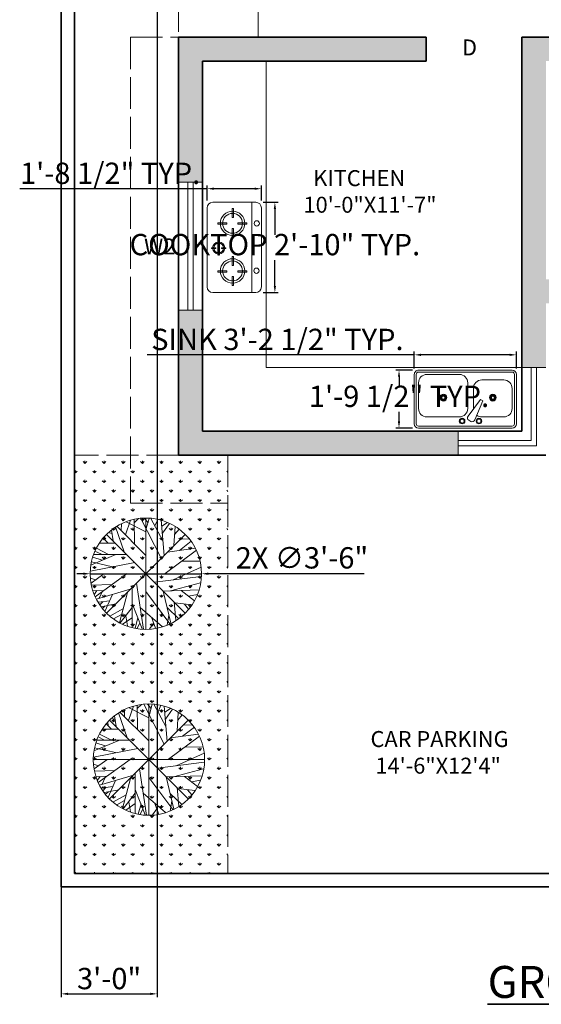
# Model space of a CAD drawing. Units: inches. Extents: x 1070 to 2371, y 645 to 1546.
# Tile 1 of 10: x 1147 to 1342, y 645 to 1014. Entities that reach past the tile are written whole.
import ezdxf

# ---------------------------------------------------------------- set-up
doc = ezdxf.new("R2010")
doc.units = ezdxf.units.IN
doc.linetypes.add('ACAD_ISO02W100', pattern=[15, 12, -3])
for name, color, linetype, lineweight in [('A-ANNO-DIMS', 2, 'Continuous', 18), ('A-ANNO-TEXT', 7, 'Continuous', 18), ('A-ANNO-TITL', 7, 'Continuous', 35), ('A-AREA-IDEN', 7, 'Continuous', 18), ('A-DOOR', 4, 'Continuous', 18), ('A-EQPM', 9, 'Continuous', 18), ('A-FLOR-CASE', 9, 'Continuous', 18), ('A-FLOR-FIXT', 9, 'Continuous', 18), ('A-GLAZ', 4, 'Continuous', 18), ('A-ROOF-OVHD', 8, 'ACAD_ISO02W100', 13), ('A-WALL', 7, 'Continuous', 35), ('C-PROP', 7, 'Continuous', 35), ('L-PLNT-BEDS-HIDN', 3, 'ACAD_ISO02W100', 13), ('L-PLNT-TREE', 94, 'Continuous', 13)]:
    doc.layers.add(name, color=color, linetype=linetype, lineweight=lineweight)
doc.layers.add('A-WALL-PATT', color=162, linetype='Continuous', lineweight=13, true_color=0x044ac3)
doc.layers.add('L-PLNT-PATT', color=85, linetype='Continuous', lineweight=13, true_color=0x58ba48)
doc.styles.get("Standard").update_dxf_attribs({"font": 'arial.ttf'})
doc.dimstyles.new('ISO-25', dxfattribs={"dimtxt": 8, "dimasz": 2.5, "dimexe": 1.25, "dimexo": 0.625, "dimtad": 1, "dimtih": 1, "dimtoh": 1, "dimdec": 1, "dimlunit": 3, "dimtxsty": 'Standard', "dimcen": 2.5, "dimadec": 0, "dimazin": 0, "dimtfac": 1, "dimtdec": 1, "dimtmove": 0, "dimatfit": 3, "dimfxl": 1, "dimarcsym": 0})

# ---------------------------------------------------------------- blocks, each defined once
blk = doc.blocks.new('A$C51B36FC3')
at = {"linetype": 'ByBlock'}
for p, q in [((0, 421.4), (0, 33)), ((15, 421.4), (15, 33)), ((767.9, 454.4), (33, 454.4)), ((767.9, 439.4), (33, 439.4)), ((325.7, 391), (261.9, 241.3)), ((357.3, 402.3), (372.7, 393.4)), ((785.9, 33), (785.9, 421.4)), ((800.9, 33), (800.9, 421.4)), ((99.1, 366.3), (271.4, 366.3)), ((281, 230.3), (378.7, 360.4)), ((447.6, 366.3), (701.8, 366.3)), ((33, 143.2), (33, 300.3)), ((171.7, 226.6), (164.2, 233.2)), ((174.6, 229.3), (168.8, 237.4)), ((178.2, 231.2), (174.5, 240.5)), ((181.4, 232.2), (179.7, 242)), ((185.3, 232.4), (185.8, 242.4)), ((189.3, 231.7), (192.3, 241.3)), ((193.1, 230.1), (198.2, 238.7)), ((196, 227.8), (203, 235)), ((261.9, 241.3), (281, 230.3)), ((337.5, 299.4), (337.5, 143.2)), ((381.5, 99.1), (381.5, 300.3)), ((560, 226.6), (552.4, 233.2)), ((562.9, 229.3), (557.1, 237.4)), ((566.5, 231.2), (562.8, 240.5)), ((569.7, 232.2), (567.9, 242)), ((573.5, 232.4), (574, 242.4)), ((577.6, 231.7), (580.5, 241.3)), ((581.3, 230.1), (586.4, 238.7)), ((584.3, 227.8), (591.2, 235)), ((767.9, 300.3), (767.9, 99.1)), ((167.7, 217.2), (157.7, 218.2)), ((167.7, 213.8), (157.8, 212.7)), ((168.5, 220.9), (159, 224.1)), ((168.6, 210), (159.2, 206.6)), ((169.7, 223.8), (161, 228.6)), ((170.1, 206.9), (161.5, 201.7)), ((172.4, 203.8), (165.3, 196.8)), ((175, 201.7), (169.3, 193.4)), ((179.3, 199.6), (176.3, 190.1)), ((184.7, 198.8), (184.8, 188.8)), ((188.6, 199.3), (191.1, 189.6)), ((192, 200.6), (196.5, 191.7)), ((195.5, 202.9), (202.1, 195.4)), ((198.3, 206.1), (206.6, 200.5)), ((199, 224.1), (207.6, 229.1)), ((200.1, 209.6), (209.5, 206)), ((200.4, 221), (209.9, 224.1)), ((201, 212.9), (210.9, 211.3)), ((201.2, 216.9), (211.2, 217.6)), ((555.9, 217.2), (546, 218.2)), ((556, 213.8), (546, 212.7)), ((556.7, 220.9), (547.2, 224.1)), ((556.8, 210), (547.4, 206.6)), ((558, 223.8), (549.2, 228.6)), ((558.3, 206.9), (549.8, 201.7)), ((560.7, 203.8), (553.6, 196.8)), ((563.2, 201.7), (557.6, 193.4)), ((567.6, 199.6), (564.5, 190.1)), ((572.9, 198.8), (573.1, 188.8)), ((576.9, 199.3), (579.4, 189.6)), ((580.3, 200.6), (584.8, 191.7)), ((583.7, 202.9), (590.3, 195.4)), ((586.6, 206.1), (594.8, 200.5)), ((587.2, 224.1), (595.9, 229.1)), ((588.4, 209.6), (597.7, 206)), ((588.6, 221), (598.1, 224.1)), ((589.3, 212.9), (599.2, 211.3)), ((589.5, 216.9), (599.4, 217.6)), ((33, 15), (767.9, 15)), ((33, 0), (767.9, 0)), ((271.4, 77.1), (99.1, 77.1)), ((701.8, 33), (447.6, 33))]:
    blk.add_line(p, q, dxfattribs=at)
for centre, radius in [((293.4, 399.4), 22), ((293.4, 399.4), 16), ((425.6, 399.4), 22), ((425.6, 399.4), 16), ((184.4, 215.6), 26.8), ((184.4, 215.6), 16.8), ((572.7, 215.6), 26.8), ((572.7, 215.6), 16.8), ((184.4, 215.6), 11.8), ((572.7, 215.6), 11.8)]:
    blk.add_circle(centre, radius, dxfattribs=at)
for centre, radius, start, end in [((33, 421.4), 33, 90, 180), ((33, 421.4), 18, 90, 180), ((346.3, 383.2), 22, 60, 159.46232), ((361.7, 374.4), 22, 320.53768, 60), ((767.9, 421.4), 33, 0, 90), ((767.9, 421.4), 18, 0, 90), ((99.1, 300.3), 66.1, 90, 180), ((271.4, 300.3), 66.1, 56.60703, 90), ((447.6, 300.3), 66.1, 90, 180), ((701.8, 300.3), 66.1, 0, 90), ((99.1, 143.2), 66.1, 180, 270), ((271.4, 143.2), 66.1, 270, 0), ((447.6, 99.1), 66.1, 180, 270), ((701.8, 99.1), 66.1, 270, 0), ((33, 33), 33, 180, 270), ((33, 33), 18, 180, 270), ((767.9, 33), 33, 270, 0), ((767.9, 33), 18, 270, 0)]:
    blk.add_arc(centre, radius, start, end, dxfattribs=at)
blk = doc.blocks.new('A$C2A3C6842')
for p, q in [((45, 432), (675, 432)), ((351.6, 363.3), (351.6, 398.9)), ((351.6, 398.9), (357.3, 398.9)), ((357.3, 398.9), (357.3, 363.3)), ((0, 45), (0, 387)), ((161.8, 346.9), (173.2, 346.9)), ((161.8, 275.6), (161.8, 346.9)), ((173.2, 346.9), (173.2, 275.6)), ((298.4, 341.9), (298.4, 336.2)), ((334, 341.9), (298.4, 341.9)), ((298.4, 336.2), (334, 336.2)), ((334, 336.2), (334, 341.9)), ((357.3, 363.3), (351.6, 363.3)), ((357.3, 318.8), (351.6, 318.8)), ((351.6, 318.8), (351.6, 283.1)), ((357.3, 283.1), (357.3, 318.8)), ((378.5, 336.2), (378.5, 341.9)), ((378.5, 341.9), (414.2, 341.9)), ((414.2, 336.2), (378.5, 336.2)), ((414.2, 341.9), (414.2, 336.2)), ((544.7, 346.9), (556.1, 346.9)), ((544.7, 275.6), (544.7, 346.9)), ((556.1, 346.9), (556.1, 275.6)), ((720, 387), (720, 45)), ((173.2, 275.6), (161.8, 275.6)), ((351.6, 283.1), (357.3, 283.1)), ((556.1, 275.6), (544.7, 275.6)), ((55.3, 232.9), (55.3, 221.5)), ((126.6, 232.9), (55.3, 232.9)), ((55.3, 221.5), (126.6, 221.5)), ((126.6, 221.5), (126.6, 232.9)), ((173.2, 186.6), (161.8, 186.6)), ((161.8, 186.6), (161.8, 115.3)), ((173.2, 115.3), (173.2, 186.6)), ((215.6, 221.5), (215.6, 232.9)), ((215.6, 232.9), (286.9, 232.9)), ((286.9, 221.5), (215.6, 221.5)), ((286.9, 232.9), (286.9, 221.5)), ((438.2, 232.9), (438.2, 221.5)), ((509.5, 232.9), (438.2, 232.9)), ((438.2, 221.5), (509.5, 221.5)), ((509.5, 221.5), (509.5, 232.9)), ((556.1, 186.6), (544.7, 186.6)), ((544.7, 186.6), (544.7, 115.3)), ((556.1, 115.3), (556.1, 186.6)), ((598.5, 232.9), (669.8, 232.9)), ((598.5, 221.5), (598.5, 232.9)), ((669.8, 221.5), (598.5, 221.5)), ((669.8, 232.9), (669.8, 221.5)), ((161.8, 115.3), (173.2, 115.3)), ((544.7, 115.3), (556.1, 115.3)), ((1.2, 76.7), (719.9, 76.7)), ((675, 0), (45, 0))]:
    blk.add_line(p, q)
at = {"extrusion": (0, -1e-16, -1)}
for centre, major_axis, start_param, end_param in [((45, 387), (31.8, 31.8), 3.926991, 5.497787), ((172.2, 229.8), (-97.3, 0.1), -0.001099, 6.282086), ((551.8, 229.8), (-97.3, 0.1), -0.001099, 6.282086), ((173.7, 39), (-14.8, 14.8), 5.497787, 11.780972)]:
    blk.add_ellipse(centre, major_axis=major_axis, ratio=1, start_param=start_param, end_param=end_param, dxfattribs=at)
at = {"extrusion": (0, 1e-16, -1)}
blk.add_ellipse((675, 387), major_axis=(-31.8, 31.8), ratio=1, start_param=0.785398, end_param=2.356194, dxfattribs=at)
at = {"extrusion": (-1e-16, -1e-16, -1)}
blk.add_ellipse((355.1, 340.4), major_axis=(48.7, 0.1), ratio=1, start_param=3.144125, end_param=9.42731, dxfattribs=at)
at = {"extrusion": (-1e-16, 0, -1)}
for centre, major_axis, start_param, end_param in [((355.1, 340.4), (-39.7, 0), -0.000334, 6.282851), ((45, 45), (-31.8, 31.8), 3.926991, 5.497787)]:
    blk.add_ellipse(centre, major_axis=major_axis, ratio=1, start_param=start_param, end_param=end_param, dxfattribs=at)
at = {"extrusion": (-1e-16, -4e-16, -1)}
for centre in [(172.2, 229.8), (551.8, 229.8)]:
    blk.add_ellipse(centre, major_axis=(-79.3, 0), ratio=1, start_param=-0.0002116186602152, end_param=6.282973688519371, dxfattribs=at)
at = {"extrusion": (2e-16, -2e-16, -1)}
blk.add_ellipse((551.4, 36.4), major_axis=(14.8, 14.8), ratio=1, start_param=3.926991, end_param=10.210176, dxfattribs=at)
at = {"extrusion": (-2e-16, 1e-16, -1)}
blk.add_ellipse((675, 45), major_axis=(31.8, 31.8), ratio=1, start_param=0.785398, end_param=2.356194, dxfattribs=at)
at = {"text_generation_flag": 4, "flags": 9}
for tag in ['XSIZE', 'YSIZE']:
    blk.add_attdef(tag, (361.3, 264.9), '', height=0.45, rotation=180, dxfattribs=at)
blk = doc.blocks.new('Tree - deciduous plan')
for p, q in [((-26.4472, 46.5894), (-26.2712, 53.8116)), ((-22.0458, 42.0753), (-16.5881, 57.6486)), ((-21.1656, 55.8436), (-0.0388, 45.0094)), ((-12.5388, 54.9406), (-7.9613, 59.4546)), ((-12.3627, 32.1443), (-12.5388, 58.7776)), ((-5.3205, 59.6806), (16.5105, 16.7963)), ((2.426, 54.9406), (-1.4472, 59.9056)), ((0, 59.9996), (0, -60)), ((0.4894, 48.6208), (3.6584, 59.6806)), ((18.2711, 35.5298), (5.419, 59.6806)), ((9.8203, 51.5549), (12.8133, 58.5516)), ((19.6795, 19.5047), (16.3344, 57.6486)), ((17.0387, 51.1035), (23.2006, 55.1666)), ((17.7429, 43.6552), (25.4894, 54.2636)), ((-40.1797, 44.558), (-36.4825, 43.2038)), ((-37.0107, 47.0408), (-35.25, 35.5298)), ((-32.6092, 50.4264), (-23.2782, 23.5674)), ((-31.2008, 51.1035), (-0.2149, 20.1818)), ((31.6513, 50.8778), (30.2429, 30.5643)), ((31.1232, 42.5267), (35.8767, 48.1693)), ((-49.8627, 32.8214), (-32.7853, 32.8214)), ((-45.8134, 38.2383), (-40.5318, 33.0471)), ((-43.8768, 36.4326), (-44.405, 40.2696)), ((42, 42), (-42, -42)), ((42, -42), (-42, 42)), ((36.2288, 25.1474), (48.9049, 35.0784)), ((37.1091, 37.1098), (46.6161, 37.5612)), ((-54.7923, 24.4702), (-47.75, 21.0847)), ((-53.2078, 27.4044), (-40.1797, 20.859)), ((54.3626, 25.3731), (20.9119, 0.3198)), ((23.3767, 23.3417), (53.3063, 27.4044)), ((-59.7219, 2.8025), (-12.0106, 12.0565)), ((-32.2571, 20.6333), (-59.1937, 9.348)), ((-58.6656, 12.7336), (-35.9543, 7.5424)), ((-57.081, 17.9248), (-47.0458, 14.7649)), ((-56.0247, 20.859), (-20.8134, 20.859)), ((38.5175, 13.4107), (58.2359, 13.6364)), ((-54.6162, -24.7335), (-20.2853, 0.0941)), ((29.3626, -6.6771), (59.4682, 7.091)), ((-60, 0), (60, 0)), ((-59.7219, -4.8714), (-54.2641, -6.6771)), ((-45.2853, -0.1316), (-59.0177, -10.0627)), ((-10.074, -10.0627), (-2.5036, -59.7178)), ((9.2922, -9.1598), (59.6443, -2.8401)), ((26.3697, -18.4138), (58.9401, -9.8369)), ((-58.4895, -12.3197), (-36.4825, -11.6426)), ((-57.081, -18.4138), (-45.2853, -17.9624)), ((-52.6797, -18.188), (-55.4966, -22.0251)), ((-53.2078, -27.442), (-16.7641, -16.6081)), ((-47.2219, -19.3166), (-50.2148, -26.3135)), ((-19.9331, -20.2194), (-28.5599, -52.721)), ((-14.8275, -15.0282), (-14.6515, -57.6865)), ((-0.0388, -19.0909), (25.8415, -53.8495)), ((18.6232, -18.6394), (26.7218, -53.3981)), ((18.7992, -18.6394), (57.3556, -17.2853)), ((38.1654, -18.188), (52.426, -29.0219)), ((-38.9472, -29.0219), (-51.4472, -30.6018)), ((-46.5177, -30.1504), (-49.5106, -33.536)), ((-35.9543, -22.4765), (-44.0529, -40.5329)), ((30.419, -30.1504), (32.3556, -50.0125)), ((31.4753, -31.279), (49.6091, -33.3103)), ((45.9119, -24.0564), (55.595, -22.2508)), ((-32.4331, -32.4075), (-48.1021, -35.5674)), ((-43.7008, -34.6645), (-46.6937, -37.373)), ((-24.6867, -37.8244), (-38.7712, -45.7241)), ((-14.6515, -36.2445), (-27.6797, -52.9467)), ((-14.6515, -32.1818), (-3.912, -59.4922)), ((-6.2008, -36.2445), (17.919, -57.0094)), ((22.8485, -36.4702), (35.3485, -48.4326)), ((41.5105, -32.6332), (46.088, -38.0501)), ((-26.2712, -43.9185), (-34.7219, -48.6583)), ((-14.6515, -47.3041), (-25.0388, -54.3009)), ((-21.5177, -45.4984), (-19.9331, -56.1065)), ((-8.4895, -47.5298), (-11.4825, -58.5893)), ((-6.3768, -52.721), (-9.3698, -58.815)), ((5.9471, -46.6269), (10.5246, -58.5893)), ((24.7852, -44.8213), (23.0246, -54.978)), ((8.4119, -53.1724), (3.8344, -59.4922))]:
    blk.add_line(p, q)
blk.add_circle((0, 0), 60)
blk = doc.blocks.new('GLAZ-CORNER')
for p, q in [((27.5, 29.5), (27.5, 2)), ((29.5, 29.5), (29.5, 0)), ((0, 2), (27.5, 2)), ((0, 0), (29.5, 0))]:
    blk.add_line(p, q)
blk = doc.blocks.new('GLAZ-48IN')
for p, q in [((0, 48), (0, 0)), ((2, 48), (2, 0))]:
    blk.add_line(p, q)
blk = doc.blocks.new('COUNTER-L-KITCHEN')
for p, q in [((0, 115), (0, 0)), ((0, 0), (96, 0))]:
    blk.add_line(p, q)
blk = doc.blocks.new('*D31')
at = {"layer": 'A-ANNO-DIMS', "color": 0, "lineweight": -2, "transparency": 16777216}
for p, q in [((1294.68, 888.47), (1194.38, 888.47)), ((1294.68, 883.35), (1294.68, 889.72)), ((1330.49, 888.47), (1297.18, 888.47)), ((1332.99, 883.35), (1332.99, 889.72))]:
    blk.add_line(p, q, dxfattribs=at)
at = {"layer": 'A-ANNO-DIMS', "color": 0, "transparency": 16777216}
for points in [[(1297.18, 888.89), (1297.18, 888.05), (1294.68, 888.47)], [(1330.49, 888.89), (1330.49, 888.05), (1332.99, 888.47)]]:
    blk.add_solid(points, dxfattribs=at)
at = {"layer": 'Defpoints', "color": 0, "transparency": 16777216}
for p in [(1294.68, 888.47), (1294.68, 882.72), (1332.99, 882.72)]:
    blk.add_point(p, dxfattribs=at)
at = {"layer": 'A-ANNO-DIMS', "color": 0, "transparency": 16777216, "insert": (1243.28, 893.23), "char_height": 8, "attachment_point": 5}
blk.add_mtext('SINK 3\'-2 1/2" TYP.', dxfattribs=at)
blk = doc.blocks.new('*D32')
at = {"layer": 'A-ANNO-DIMS', "color": 0, "lineweight": -2, "transparency": 16777216}
for p, q in [((1294.06, 882.72), (1287.69, 882.72)), ((1288.94, 880.22), (1288.94, 876.62)), ((1288.94, 863.49), (1288.94, 867.09)), ((1294.06, 860.99), (1287.69, 860.99))]:
    blk.add_line(p, q, dxfattribs=at)
at = {"layer": 'A-ANNO-DIMS', "color": 0, "transparency": 16777216}
for points in [[(1288.52, 880.22), (1289.35, 880.22), (1288.94, 882.72)], [(1288.52, 863.49), (1289.35, 863.49), (1288.94, 860.99)]]:
    blk.add_solid(points, dxfattribs=at)
at = {"layer": 'Defpoints', "color": 0, "transparency": 16777216}
for p in [(1294.68, 882.72), (1288.94, 860.99), (1294.68, 860.99)]:
    blk.add_point(p, dxfattribs=at)
at = {"layer": 'A-ANNO-DIMS', "color": 0, "transparency": 16777216, "insert": (1288.94, 871.86), "char_height": 8, "attachment_point": 5}
blk.add_mtext('1\'-9 1/2" TYP.', dxfattribs=at)
blk = doc.blocks.new('*D33')
at = {"layer": 'A-ANNO-DIMS', "color": 0, "lineweight": -2, "transparency": 16777216}
for p, q in [((1237.88, 945.76), (1243.59, 945.76)), ((1242.34, 943.26), (1242.34, 933.58)), ((1242.34, 914.38), (1242.34, 924.05)), ((1237.88, 911.88), (1243.59, 911.88))]:
    blk.add_line(p, q, dxfattribs=at)
at = {"layer": 'A-ANNO-DIMS', "color": 0, "transparency": 16777216}
for points in [[(1241.92, 943.26), (1242.76, 943.26), (1242.34, 945.76)], [(1241.92, 914.38), (1242.76, 914.38), (1242.34, 911.88)]]:
    blk.add_solid(points, dxfattribs=at)
at = {"layer": 'Defpoints', "color": 0, "transparency": 16777216}
for p in [(1237.26, 945.76), (1242.34, 945.76), (1237.26, 911.88)]:
    blk.add_point(p, dxfattribs=at)
at = {"layer": 'A-ANNO-DIMS', "color": 0, "transparency": 16777216, "insert": (1242.34, 928.82), "char_height": 8, "attachment_point": 5}
blk.add_mtext('COOKTOP 2\'-10" TYP.', dxfattribs=at)
blk = doc.blocks.new('*D34')
at = {"layer": 'A-ANNO-DIMS', "color": 0, "lineweight": -2, "transparency": 16777216}
for p, q in [((1216.93, 950.84), (1146.53, 950.84)), ((1216.93, 946.38), (1216.93, 952.09)), ((1234.76, 950.84), (1219.43, 950.84)), ((1237.26, 946.38), (1237.26, 952.09))]:
    blk.add_line(p, q, dxfattribs=at)
at = {"layer": 'A-ANNO-DIMS', "color": 0, "transparency": 16777216}
for points in [[(1219.43, 951.26), (1219.43, 950.42), (1216.93, 950.84)], [(1234.76, 951.26), (1234.76, 950.42), (1237.26, 950.84)]]:
    blk.add_solid(points, dxfattribs=at)
at = {"layer": 'Defpoints', "color": 0, "transparency": 16777216}
for p in [(1216.93, 950.84), (1216.93, 945.76), (1237.26, 945.76)]:
    blk.add_point(p, dxfattribs=at)
at = {"layer": 'A-ANNO-DIMS', "color": 0, "transparency": 16777216, "insert": (1180.48, 955.6), "char_height": 8, "attachment_point": 5}
blk.add_mtext('1\'-8 1/2" TYP.', dxfattribs=at)
blk = doc.blocks.new('*D47')
at = {"layer": 'A-ANNO-DIMS', "color": 0, "lineweight": -2, "transparency": 16777216}
for p, q in [((1162.11, 1408.15), (1162.11, 647.32)), ((1198.11, 1342.15), (1198.11, 647.32)), ((1164.61, 648.57), (1195.61, 648.57))]:
    blk.add_line(p, q, dxfattribs=at)
at = {"layer": 'A-ANNO-DIMS', "color": 0, "transparency": 16777216}
for points in [[(1164.61, 648.99), (1164.61, 648.16), (1162.11, 648.57)], [(1195.61, 648.99), (1195.61, 648.16), (1198.11, 648.57)]]:
    blk.add_solid(points, dxfattribs=at)
at = {"layer": 'Defpoints', "color": 0, "transparency": 16777216}
for p in [(1162.11, 1408.77), (1198.11, 1342.77), (1198.11, 648.57)]:
    blk.add_point(p, dxfattribs=at)
at = {"layer": 'A-ANNO-DIMS', "color": 0, "transparency": 16777216, "insert": (1180.11, 653.28), "char_height": 8, "attachment_point": 5}
blk.add_mtext('3\'-0"', dxfattribs=at)
blk = doc.blocks.new('*D69')
at = {"layer": 'A-ANNO-DIMS', "color": 0, "lineweight": -2, "transparency": 16777216}
for p, q in [((1170.48, 806.29), (1167.98, 806.29)), ((1172.98, 806.29), (1214.81, 806.29)), ((1228.43, 806.29), (1217.31, 806.29)), ((1275.92, 806.29), (1228.43, 806.29))]:
    blk.add_line(p, q, dxfattribs=at)
at = {"layer": 'A-ANNO-DIMS', "color": 0, "transparency": 16777216}
for points in [[(1170.48, 806.7), (1170.48, 805.87), (1172.98, 806.29)], [(1217.31, 806.7), (1217.31, 805.87), (1214.81, 806.29)]]:
    blk.add_solid(points, dxfattribs=at)
at = {"layer": 'Defpoints', "color": 0, "transparency": 16777216}
for p in [(1172.98, 806.29), (1214.81, 806.29)]:
    blk.add_point(p, dxfattribs=at)
at = {"layer": 'A-ANNO-DIMS', "color": 0, "transparency": 16777216, "insert": (1252.49, 811.22), "char_height": 8, "attachment_point": 5}
blk.add_mtext('2X ∅3\'-6"', dxfattribs=at)

msp = doc.modelspace()

# ---------------------------------------------------------------- hatches: boundary and pattern name
at = {"layer": 'A-WALL-PATT'}
h = msp.add_hatch(color=256, dxfattribs=at)
h.dxf.hatch_style = 1
h.paths.add_polyline_path([(1502.11, 813.77), (1461.11, 813.77), (1461.11, 804.77), (1502.11, 804.77)])
h.paths.add_polyline_path([(1344.11, 998.77), (1359.11, 998.77), (1359.11, 1007.77), (1335.11, 1007.77), (1335.11, 883.77), (1344.11, 883.77), (1344.11, 907.77), (1359.11, 907.77), (1359.11, 916.77), (1344.11, 916.77)])
h.paths.add_polyline_path([(1311.11, 859.77), (1215.11, 859.77), (1215.11, 905.27), (1206.11, 905.27), (1206.11, 850.77), (1311.11, 850.77)])
h.paths.add_polyline_path([(1299.11, 1007.77), (1206.11, 1007.77), (1206.11, 953.27), (1215.11, 953.27), (1215.11, 998.77), (1299.11, 998.77)])
at = {"layer": 'L-PLNT-PATT'}
h = msp.add_hatch(dxfattribs=at)
h.set_pattern_fill('GRASS', color=256, scale=0.2)
h.paths.add_polyline_path([(1224.73, 850.77), (1206.11, 850.77), (1167.11, 850.77), (1167.11, 693.77), (1224.73, 693.77)])

# ---------------------------------------------------------------- linework, layer by layer
at = {"layer": 'A-DOOR'}
msp.add_line((1236.11, 1043.77), (1236.11, 1007.77), dxfattribs=at)
at = {"layer": 'A-GLAZ'}
for p, q in [((1215.11, 953.27), (1206.11, 953.27)), ((1215.11, 905.27), (1206.11, 905.27)), ((1335.11, 883.77), (1344.11, 883.77)), ((1311.11, 859.77), (1311.11, 850.77))]:
    msp.add_line(p, q, dxfattribs=at)
at = {"layer": 'A-ROOF-OVHD'}
for p, q in [((1206.11, 1171.77), (1206.11, 1007.77)), ((1188.11, 1007.77), (1206.11, 1007.77)), ((1188.11, 1007.77), (1188.11, 832.77)), ((1188.11, 832.77), (1224.73, 832.77))]:
    msp.add_line(p, q, dxfattribs=at)
at = {"layer": 'A-WALL'}
for p, q in [((1206.11, 1007.77), (1206.11, 850.77)), ((1206.11, 1007.77), (1299.11, 1007.77)), ((1299.11, 1007.77), (1299.11, 998.77)), ((1335.11, 1007.77), (1335.11, 859.77)), ((1335.11, 1007.77), (1359.11, 1007.77)), ((1215.11, 998.77), (1215.11, 859.77)), ((1215.11, 998.77), (1299.11, 998.77)), ((1215.11, 859.77), (1335.11, 859.77)), ((1206.11, 850.77), (1344.11, 850.77))]:
    msp.add_line(p, q, dxfattribs=at)
at = {"layer": 'C-PROP'}
for p, q in [((1162.11, 1408.77), (1162.11, 688.77)), ((1167.11, 1403.77), (1167.11, 693.77)), ((1167.11, 693.77), (1637.11, 693.77)), ((1162.11, 688.77), (1642.11, 688.77))]:
    msp.add_line(p, q, dxfattribs=at)
at = {"layer": 'L-PLNT-BEDS-HIDN'}
for p, q in [((1206.11, 850.77), (1167.11, 850.77)), ((1224.73, 850.77), (1224.73, 693.77))]:
    msp.add_line(p, q, dxfattribs=at)

# ---------------------------------------------------------------- block references
at = {"layer": 'A-EQPM', "xscale": 0.0470524325747904, "yscale": 0.0470524325747904, "zscale": 0.0470524325747904, "rotation": 90}
msp.add_blockref('A$C2A3C6842', (1237.26, 911.88), dxfattribs=at)
at = {"layer": 'A-FLOR-CASE'}
msp.add_blockref('COUNTER-L-KITCHEN', (1239.11, 883.77), dxfattribs=at)
at = {"layer": 'A-FLOR-FIXT', "xscale": 0.0478318492028633, "yscale": 0.0478318492028633, "zscale": 0.0478318492028633, "rotation": 180}
msp.add_blockref('A$C51B36FC3', (1332.99, 882.72), dxfattribs=at)
at = {"layer": 'A-GLAZ'}
for name, p in [('GLAZ-48IN', (1209.61, 905.27)), ('GLAZ-CORNER', (1311.11, 854.27))]:
    msp.add_blockref(name, p, dxfattribs=at)
at = {"layer": 'L-PLNT-TREE', "xscale": 0.3485724194044117, "yscale": 0.3485724194044117, "zscale": 0.3485724194044117}
for p in [(1193.9, 806.29), (1195.05, 736.51)]:
    msp.add_blockref('Tree - deciduous plan', p, dxfattribs=at)

# ---------------------------------------------------------------- texts
at = {"layer": 'A-ANNO-TEXT', "char_height": 6, "attachment_point": 1}
for s, insert in [('D', (1312.59, 1006.87)), ('W2', (1193.23, 932.15))]:
    msp.add_mtext_dynamic_manual_height_columns(s, width=20.5094, gutter_width=12.5, heights=[0], dxfattribs=dict(at, insert=insert))
at = {"layer": 'A-ANNO-TITL', "insert": (1322.21, 659.05), "char_height": 12, "attachment_point": 1}
msp.add_mtext_dynamic_manual_height_columns('{\\LGROUNG FLOOR }', width=357.2187, gutter_width=12.5, heights=[0], dxfattribs=at)
at = {"layer": 'A-AREA-IDEN', "char_height": 6, "attachment_point": 1}
for s, width, insert in [('   KITCHEN\\P 10\'-0"X11\'-7"', 97.1991, (1251.25, 957.82)), ('CAR PARKING\\P 14\'-6"X12\'4"', 119.0122, (1278.24, 747.24))]:
    msp.add_mtext_dynamic_manual_height_columns(s, width=width, gutter_width=12.5, heights=[0], dxfattribs=dict(at, insert=insert))

# ---------------------------------------------------------------- dimensions: what is measured, and where the dimension line sits
at = {"layer": 'A-ANNO-DIMS'}
dim = msp.add_linear_dim(base=(1198.11, 648.57), p1=(1162.11, 1408.77), p2=(1198.11, 1342.77), dimstyle='ISO-25', override={"dimdec": 1, "dimlfac": 1, "dimrnd": 0, "dimzin": 1, "dimdsep": 46, "dimlunit": 4, "dimfrac": 2}, dxfattribs=at)
dim.commit()
dim.dimension.update_dxf_attribs({"geometry": '*D47', "text_midpoint": (1180.11, 653.28)})
for base, p1, p2, angle, text, picture, middle in [((1216.93, 950.84), (1237.26, 945.76), (1216.93, 945.76), 180, '<> TYP.', '*D34', (1180.48, 955.6)), ((1242.34, 945.76), (1237.26, 911.88), (1237.26, 945.76), 90, 'COOKTOP <> TYP.', '*D33', (1242.34, 928.82)), ((1294.68, 888.47), (1332.99, 882.72), (1294.68, 882.72), 180, 'SINK <> TYP.', '*D31', (1243.28, 893.23)), ((1288.94, 860.99), (1294.68, 882.72), (1294.68, 860.99), 270, '<> TYP.', '*D32', (1288.94, 871.86))]:
    dim = msp.add_linear_dim(base=base, p1=p1, p2=p2, angle=angle, text=text, dimstyle='ISO-25', override={"dimdec": 1, "dimlfac": 1, "dimrnd": 0, "dimzin": 1, "dimdsep": 46, "dimlunit": 4, "dimfrac": 2}, dxfattribs=at)
    dim.commit()
    dim.dimension.update_dxf_attribs({"geometry": picture, "text_midpoint": middle})
dim = msp.add_diameter_dim_2p(p1=(1172.98, 806.29), p2=(1214.81, 806.29), text='2X <>', dimstyle='ISO-25', override={"dimdec": 1, "dimlfac": 1, "dimrnd": 0, "dimzin": 1, "dimdsep": 46, "dimlunit": 4, "dimfrac": 2}, dxfattribs=at)
dim.commit()
dim.dimension.update_dxf_attribs({"geometry": '*D69', "text_midpoint": (1228.43, 806.29)})

doc.saveas('drawing.dxf')
